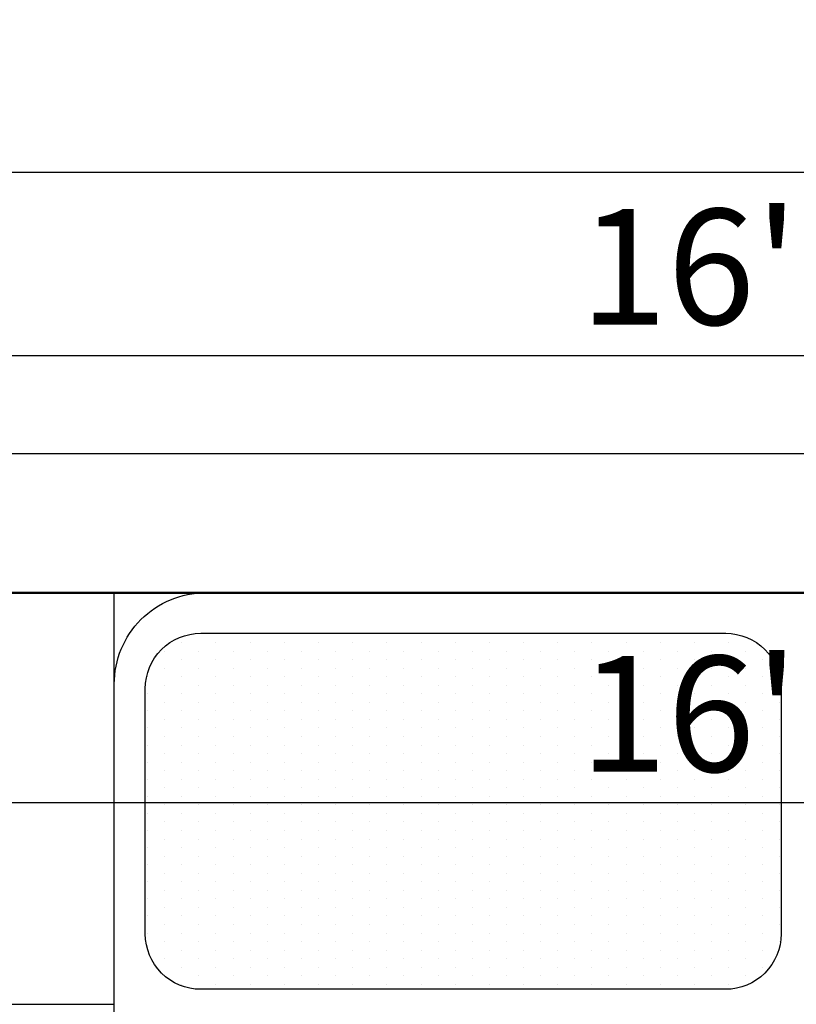
# Model space of a CAD drawing. Units: inches. Extents: x 3064 to 19385, y 846 to 15425.
# Tile 89 of 108: x 7305 to 7338, y 1373 to 1415. Entities that reach past the tile are written whole.
import ezdxf

# ---------------------------------------------------------------- set-up
doc = ezdxf.new("R2010")
doc.units = ezdxf.units.IN
for name, color, linetype, lineweight in [('A-ANNO-DIMS', 2, 'Continuous', 18), ('A-FLOR-FIXT', 9, 'Continuous', 18), ('A-WALL', 7, 'Continuous', 50), ('C-PROP', 6, 'Continuous', 25)]:
    doc.layers.add(name, color=color, linetype=linetype, lineweight=lineweight)
doc.layers.add('BLOCK', color=6, linetype='Continuous')
doc.styles.get("Standard").update_dxf_attribs({"font": 'arial.ttf'})
doc.dimstyles.new('ISO-25', dxfattribs={"dimtxt": 9, "dimasz": 2.5, "dimexe": 1.25, "dimexo": 0.625, "dimtad": 1, "dimdec": 1, "dimlunit": 3, "dimtxsty": 'Standard', "dimcen": 2.5, "dimadec": 0, "dimazin": 0, "dimtfac": 1, "dimtdec": 1, "dimtmove": 0, "dimatfit": 3, "dimfxl": 1, "dimarcsym": 0})

# ---------------------------------------------------------------- blocks, each defined once
blk = doc.blocks.new('*D294')
at = {"layer": 'A-ANNO-DIMS', "color": 0, "lineweight": -2, "transparency": 16777216}
for p, q in [((7240.705, 1396.965), (7240.705, 1401.844)), ((7435.705, 1396.965), (7435.705, 1401.844)), ((7243.205, 1400.594), (7433.205, 1400.594))]:
    blk.add_line(p, q, dxfattribs=at)
at = {"layer": 'A-ANNO-DIMS', "color": 0, "transparency": 16777216}
for points in [[(7243.205, 1401.011), (7243.205, 1400.178), (7240.705, 1400.594)], [(7433.205, 1401.011), (7433.205, 1400.178), (7435.705, 1400.594)]]:
    blk.add_solid(points, dxfattribs=at)
at = {"layer": 'Defpoints', "color": 0, "transparency": 16777216}
for p in [(7435.705, 1400.594), (7240.705, 1396.34), (7435.705, 1396.34)]:
    blk.add_point(p, dxfattribs=at)
at = {"layer": 'A-ANNO-DIMS', "color": 0, "transparency": 16777216, "insert": (7338.205, 1403.774), "char_height": 5, "attachment_point": 5}
blk.add_mtext('16\'-3"', dxfattribs=at)
blk = doc.blocks.new('*D315')
at = {"layer": 'A-ANNO-DIMS', "color": 0, "lineweight": -2, "transparency": 16777216}
for p, q in [((7099.705, 1396.965), (7099.705, 1409.763)), ((7441.705, 1396.965), (7441.705, 1409.763)), ((7102.205, 1408.513), (7439.205, 1408.513))]:
    blk.add_line(p, q, dxfattribs=at)
at = {"layer": 'A-ANNO-DIMS', "color": 0, "transparency": 16777216}
for points in [[(7102.205, 1408.929), (7102.205, 1408.096), (7099.705, 1408.513)], [(7439.205, 1408.929), (7439.205, 1408.096), (7441.705, 1408.513)]]:
    blk.add_solid(points, dxfattribs=at)
at = {"layer": 'Defpoints', "color": 0, "transparency": 16777216}
for p in [(7441.705, 1408.513), (7099.705, 1396.34), (7441.705, 1396.34)]:
    blk.add_point(p, dxfattribs=at)
at = {"layer": 'A-ANNO-DIMS', "color": 0, "transparency": 16777216, "insert": (7270.705, 1411.691), "char_height": 5, "attachment_point": 5}
blk.add_mtext('28\'-6"', dxfattribs=at)
blk = doc.blocks.new('*D290')
at = {"layer": 'A-ANNO-DIMS', "color": 0, "lineweight": -2, "transparency": 16777216}
for p, q in [((7240.705, 1389.715), (7240.705, 1380.039)), ((7435.705, 1389.715), (7435.705, 1380.039)), ((7243.205, 1381.289), (7433.205, 1381.289))]:
    blk.add_line(p, q, dxfattribs=at)
at = {"layer": 'A-ANNO-DIMS', "color": 0, "transparency": 16777216}
for points in [[(7243.205, 1381.705), (7243.205, 1380.872), (7240.705, 1381.289)], [(7433.205, 1381.705), (7433.205, 1380.872), (7435.705, 1381.289)]]:
    blk.add_solid(points, dxfattribs=at)
at = {"layer": 'Defpoints', "color": 0, "transparency": 16777216}
for p in [(7240.705, 1390.34), (7435.705, 1390.34), (7435.705, 1381.289)]:
    blk.add_point(p, dxfattribs=at)
at = {"layer": 'A-ANNO-DIMS', "color": 0, "transparency": 16777216, "insert": (7338.205, 1384.468), "char_height": 5, "attachment_point": 5}
blk.add_mtext('16\'-3"', dxfattribs=at)
blk = doc.blocks.new('*X7')
at = {"color": 0}
for p, q in [((266.25, 456.9375), (266.25, 456.9375)), ((266.4375, 457.03125), (266.4375, 457.03125)), ((266.625, 456.9375), (266.625, 456.9375)), ((266.8125, 457.03125), (266.8125, 457.03125)), ((267, 456.9375), (267, 456.9375)), ((267.1875, 457.03125), (267.1875, 457.03125)), ((267.375, 456.9375), (267.375, 456.9375)), ((267.5625, 457.03125), (267.5625, 457.03125)), ((267.75, 456.9375), (267.75, 456.9375)), ((267.9375, 457.03125), (267.9375, 457.03125)), ((268.125, 456.9375), (268.125, 456.9375)), ((268.3125, 457.03125), (268.3125, 457.03125)), ((268.5, 456.9375), (268.5, 456.9375)), ((268.6875, 457.03125), (268.6875, 457.03125)), ((268.875, 456.9375), (268.875, 456.9375)), ((269.0625, 457.03125), (269.0625, 457.03125)), ((269.25, 456.9375), (269.25, 456.9375)), ((269.4375, 457.03125), (269.4375, 457.03125)), ((269.625, 456.9375), (269.625, 456.9375)), ((269.8125, 457.03125), (269.8125, 457.03125)), ((270, 456.9375), (270, 456.9375)), ((270.1875, 457.03125), (270.1875, 457.03125)), ((270.375, 456.9375), (270.375, 456.9375)), ((270.5625, 457.03125), (270.5625, 457.03125)), ((270.75, 456.9375), (270.75, 456.9375)), ((270.9375, 457.03125), (270.9375, 457.03125)), ((271.125, 456.9375), (271.125, 456.9375)), ((271.3125, 457.03125), (271.3125, 457.03125)), ((271.5, 456.9375), (271.5, 456.9375)), ((271.6875, 457.03125), (271.6875, 457.03125)), ((271.875, 456.9375), (271.875, 456.9375)), ((272.0625, 457.03125), (272.0625, 457.03125)), ((272.25, 456.9375), (272.25, 456.9375)), ((266.0625, 456.84375), (266.0625, 456.84375)), ((266.4375, 456.84375), (266.4375, 456.84375)), ((266.8125, 456.84375), (266.8125, 456.84375)), ((267.1875, 456.84375), (267.1875, 456.84375)), ((267.5625, 456.84375), (267.5625, 456.84375)), ((267.9375, 456.84375), (267.9375, 456.84375)), ((268.3125, 456.84375), (268.3125, 456.84375)), ((268.6875, 456.84375), (268.6875, 456.84375)), ((269.0625, 456.84375), (269.0625, 456.84375)), ((269.4375, 456.84375), (269.4375, 456.84375)), ((269.8125, 456.84375), (269.8125, 456.84375)), ((270.1875, 456.84375), (270.1875, 456.84375)), ((270.5625, 456.84375), (270.5625, 456.84375)), ((270.9375, 456.84375), (270.9375, 456.84375)), ((271.3125, 456.84375), (271.3125, 456.84375)), ((271.6875, 456.84375), (271.6875, 456.84375)), ((272.0625, 456.84375), (272.0625, 456.84375)), ((272.4375, 456.84375), (272.4375, 456.84375)), ((266.25, 456.75), (266.25, 456.75)), ((266.625, 456.75), (266.625, 456.75)), ((267, 456.75), (267, 456.75)), ((267.375, 456.75), (267.375, 456.75)), ((267.75, 456.75), (267.75, 456.75)), ((268.125, 456.75), (268.125, 456.75)), ((268.5, 456.75), (268.5, 456.75)), ((268.875, 456.75), (268.875, 456.75)), ((269.25, 456.75), (269.25, 456.75)), ((269.625, 456.75), (269.625, 456.75)), ((270, 456.75), (270, 456.75)), ((270.375, 456.75), (270.375, 456.75)), ((270.75, 456.75), (270.75, 456.75)), ((271.125, 456.75), (271.125, 456.75)), ((271.5, 456.75), (271.5, 456.75)), ((271.875, 456.75), (271.875, 456.75)), ((272.25, 456.75), (272.25, 456.75)), ((272.625, 456.75), (272.625, 456.75)), ((266.0625, 456.65625), (266.0625, 456.65625)), ((266.4375, 456.65625), (266.4375, 456.65625)), ((266.8125, 456.65625), (266.8125, 456.65625)), ((267.1875, 456.65625), (267.1875, 456.65625)), ((267.5625, 456.65625), (267.5625, 456.65625)), ((267.9375, 456.65625), (267.9375, 456.65625)), ((268.3125, 456.65625), (268.3125, 456.65625)), ((268.6875, 456.65625), (268.6875, 456.65625)), ((269.0625, 456.65625), (269.0625, 456.65625)), ((269.4375, 456.65625), (269.4375, 456.65625)), ((269.8125, 456.65625), (269.8125, 456.65625)), ((270.1875, 456.65625), (270.1875, 456.65625)), ((270.5625, 456.65625), (270.5625, 456.65625)), ((270.9375, 456.65625), (270.9375, 456.65625)), ((271.3125, 456.65625), (271.3125, 456.65625)), ((271.6875, 456.65625), (271.6875, 456.65625)), ((272.0625, 456.65625), (272.0625, 456.65625)), ((272.4375, 456.65625), (272.4375, 456.65625)), ((265.875, 456.5625), (265.875, 456.5625)), ((266.25, 456.5625), (266.25, 456.5625)), ((266.625, 456.5625), (266.625, 456.5625)), ((267, 456.5625), (267, 456.5625)), ((267.375, 456.5625), (267.375, 456.5625)), ((267.75, 456.5625), (267.75, 456.5625)), ((268.125, 456.5625), (268.125, 456.5625)), ((268.5, 456.5625), (268.5, 456.5625)), ((268.875, 456.5625), (268.875, 456.5625)), ((269.25, 456.5625), (269.25, 456.5625)), ((269.625, 456.5625), (269.625, 456.5625)), ((270, 456.5625), (270, 456.5625)), ((270.375, 456.5625), (270.375, 456.5625)), ((270.75, 456.5625), (270.75, 456.5625)), ((271.125, 456.5625), (271.125, 456.5625)), ((271.5, 456.5625), (271.5, 456.5625)), ((271.875, 456.5625), (271.875, 456.5625)), ((272.25, 456.5625), (272.25, 456.5625)), ((272.625, 456.5625), (272.625, 456.5625)), ((266.0625, 456.46875), (266.0625, 456.46875)), ((266.4375, 456.46875), (266.4375, 456.46875)), ((266.8125, 456.46875), (266.8125, 456.46875)), ((267.1875, 456.46875), (267.1875, 456.46875)), ((267.5625, 456.46875), (267.5625, 456.46875)), ((267.9375, 456.46875), (267.9375, 456.46875)), ((268.3125, 456.46875), (268.3125, 456.46875)), ((268.6875, 456.46875), (268.6875, 456.46875)), ((269.0625, 456.46875), (269.0625, 456.46875)), ((269.4375, 456.46875), (269.4375, 456.46875)), ((269.8125, 456.46875), (269.8125, 456.46875)), ((270.1875, 456.46875), (270.1875, 456.46875)), ((270.5625, 456.46875), (270.5625, 456.46875)), ((270.9375, 456.46875), (270.9375, 456.46875)), ((271.3125, 456.46875), (271.3125, 456.46875)), ((271.6875, 456.46875), (271.6875, 456.46875)), ((272.0625, 456.46875), (272.0625, 456.46875)), ((272.4375, 456.46875), (272.4375, 456.46875)), ((272.8125, 456.46875), (272.8125, 456.46875)), ((265.875, 456.375), (265.875, 456.375)), ((266.25, 456.375), (266.25, 456.375)), ((266.625, 456.375), (266.625, 456.375)), ((267, 456.375), (267, 456.375)), ((267.375, 456.375), (267.375, 456.375)), ((267.75, 456.375), (267.75, 456.375)), ((268.125, 456.375), (268.125, 456.375)), ((268.5, 456.375), (268.5, 456.375)), ((268.875, 456.375), (268.875, 456.375)), ((269.25, 456.375), (269.25, 456.375)), ((269.625, 456.375), (269.625, 456.375)), ((270, 456.375), (270, 456.375)), ((270.375, 456.375), (270.375, 456.375)), ((270.75, 456.375), (270.75, 456.375)), ((271.125, 456.375), (271.125, 456.375)), ((271.5, 456.375), (271.5, 456.375)), ((271.875, 456.375), (271.875, 456.375)), ((272.25, 456.375), (272.25, 456.375)), ((272.625, 456.375), (272.625, 456.375)), ((265.875, 456.1875), (265.875, 456.1875)), ((266.0625, 456.28125), (266.0625, 456.28125)), ((266.25, 456.1875), (266.25, 456.1875)), ((266.4375, 456.28125), (266.4375, 456.28125)), ((266.625, 456.1875), (266.625, 456.1875)), ((266.8125, 456.28125), (266.8125, 456.28125)), ((267, 456.1875), (267, 456.1875)), ((267.1875, 456.28125), (267.1875, 456.28125)), ((267.375, 456.1875), (267.375, 456.1875)), ((267.5625, 456.28125), (267.5625, 456.28125)), ((267.75, 456.1875), (267.75, 456.1875)), ((267.9375, 456.28125), (267.9375, 456.28125)), ((268.125, 456.1875), (268.125, 456.1875)), ((268.3125, 456.28125), (268.3125, 456.28125)), ((268.5, 456.1875), (268.5, 456.1875)), ((268.6875, 456.28125), (268.6875, 456.28125)), ((268.875, 456.1875), (268.875, 456.1875)), ((269.0625, 456.28125), (269.0625, 456.28125)), ((269.25, 456.1875), (269.25, 456.1875)), ((269.4375, 456.28125), (269.4375, 456.28125)), ((269.625, 456.1875), (269.625, 456.1875)), ((269.8125, 456.28125), (269.8125, 456.28125)), ((270, 456.1875), (270, 456.1875)), ((270.1875, 456.28125), (270.1875, 456.28125)), ((270.375, 456.1875), (270.375, 456.1875)), ((270.5625, 456.28125), (270.5625, 456.28125)), ((270.75, 456.1875), (270.75, 456.1875)), ((270.9375, 456.28125), (270.9375, 456.28125)), ((271.125, 456.1875), (271.125, 456.1875)), ((271.3125, 456.28125), (271.3125, 456.28125)), ((271.5, 456.1875), (271.5, 456.1875)), ((271.6875, 456.28125), (271.6875, 456.28125)), ((271.875, 456.1875), (271.875, 456.1875)), ((272.0625, 456.28125), (272.0625, 456.28125)), ((272.25, 456.1875), (272.25, 456.1875)), ((272.4375, 456.28125), (272.4375, 456.28125)), ((272.625, 456.1875), (272.625, 456.1875)), ((272.8125, 456.28125), (272.8125, 456.28125)), ((266.0625, 456.09375), (266.0625, 456.09375)), ((266.4375, 456.09375), (266.4375, 456.09375)), ((266.8125, 456.09375), (266.8125, 456.09375)), ((267.1875, 456.09375), (267.1875, 456.09375)), ((267.5625, 456.09375), (267.5625, 456.09375)), ((267.9375, 456.09375), (267.9375, 456.09375)), ((268.3125, 456.09375), (268.3125, 456.09375)), ((268.6875, 456.09375), (268.6875, 456.09375)), ((269.0625, 456.09375), (269.0625, 456.09375)), ((269.4375, 456.09375), (269.4375, 456.09375)), ((269.8125, 456.09375), (269.8125, 456.09375)), ((270.1875, 456.09375), (270.1875, 456.09375)), ((270.5625, 456.09375), (270.5625, 456.09375)), ((270.9375, 456.09375), (270.9375, 456.09375)), ((271.3125, 456.09375), (271.3125, 456.09375)), ((271.6875, 456.09375), (271.6875, 456.09375)), ((272.0625, 456.09375), (272.0625, 456.09375)), ((272.4375, 456.09375), (272.4375, 456.09375)), ((272.8125, 456.09375), (272.8125, 456.09375)), ((265.875, 456), (265.875, 456)), ((266.25, 456), (266.25, 456)), ((266.625, 456), (266.625, 456)), ((267, 456), (267, 456)), ((267.375, 456), (267.375, 456)), ((267.75, 456), (267.75, 456)), ((268.125, 456), (268.125, 456)), ((268.5, 456), (268.5, 456)), ((268.875, 456), (268.875, 456)), ((269.25, 456), (269.25, 456)), ((269.625, 456), (269.625, 456)), ((270, 456), (270, 456)), ((270.375, 456), (270.375, 456)), ((270.75, 456), (270.75, 456)), ((271.125, 456), (271.125, 456)), ((271.5, 456), (271.5, 456)), ((271.875, 456), (271.875, 456)), ((272.25, 456), (272.25, 456)), ((272.625, 456), (272.625, 456)), ((266.0625, 455.90625), (266.0625, 455.90625)), ((266.4375, 455.90625), (266.4375, 455.90625)), ((266.8125, 455.90625), (266.8125, 455.90625)), ((267.1875, 455.90625), (267.1875, 455.90625)), ((267.5625, 455.90625), (267.5625, 455.90625)), ((267.9375, 455.90625), (267.9375, 455.90625)), ((268.3125, 455.90625), (268.3125, 455.90625)), ((268.6875, 455.90625), (268.6875, 455.90625)), ((269.0625, 455.90625), (269.0625, 455.90625)), ((269.4375, 455.90625), (269.4375, 455.90625)), ((269.8125, 455.90625), (269.8125, 455.90625)), ((270.1875, 455.90625), (270.1875, 455.90625)), ((270.5625, 455.90625), (270.5625, 455.90625)), ((270.9375, 455.90625), (270.9375, 455.90625)), ((271.3125, 455.90625), (271.3125, 455.90625)), ((271.6875, 455.90625), (271.6875, 455.90625)), ((272.0625, 455.90625), (272.0625, 455.90625)), ((272.4375, 455.90625), (272.4375, 455.90625)), ((272.8125, 455.90625), (272.8125, 455.90625)), ((265.875, 455.8125), (265.875, 455.8125)), ((266.25, 455.8125), (266.25, 455.8125)), ((266.625, 455.8125), (266.625, 455.8125)), ((267, 455.8125), (267, 455.8125)), ((267.375, 455.8125), (267.375, 455.8125)), ((267.75, 455.8125), (267.75, 455.8125)), ((268.125, 455.8125), (268.125, 455.8125)), ((268.5, 455.8125), (268.5, 455.8125)), ((268.875, 455.8125), (268.875, 455.8125)), ((269.25, 455.8125), (269.25, 455.8125)), ((269.625, 455.8125), (269.625, 455.8125)), ((270, 455.8125), (270, 455.8125)), ((270.375, 455.8125), (270.375, 455.8125)), ((270.75, 455.8125), (270.75, 455.8125)), ((271.125, 455.8125), (271.125, 455.8125)), ((271.5, 455.8125), (271.5, 455.8125)), ((271.875, 455.8125), (271.875, 455.8125)), ((272.25, 455.8125), (272.25, 455.8125)), ((272.625, 455.8125), (272.625, 455.8125)), ((266.0625, 455.71875), (266.0625, 455.71875)), ((266.4375, 455.71875), (266.4375, 455.71875)), ((266.8125, 455.71875), (266.8125, 455.71875)), ((267.1875, 455.71875), (267.1875, 455.71875)), ((267.5625, 455.71875), (267.5625, 455.71875)), ((267.9375, 455.71875), (267.9375, 455.71875)), ((268.3125, 455.71875), (268.3125, 455.71875)), ((268.6875, 455.71875), (268.6875, 455.71875)), ((269.0625, 455.71875), (269.0625, 455.71875)), ((269.4375, 455.71875), (269.4375, 455.71875)), ((269.8125, 455.71875), (269.8125, 455.71875)), ((270.1875, 455.71875), (270.1875, 455.71875)), ((270.5625, 455.71875), (270.5625, 455.71875)), ((270.9375, 455.71875), (270.9375, 455.71875)), ((271.3125, 455.71875), (271.3125, 455.71875)), ((271.6875, 455.71875), (271.6875, 455.71875)), ((272.0625, 455.71875), (272.0625, 455.71875)), ((272.4375, 455.71875), (272.4375, 455.71875)), ((272.8125, 455.71875), (272.8125, 455.71875)), ((265.875, 455.625), (265.875, 455.625)), ((266.0625, 455.53125), (266.0625, 455.53125)), ((266.25, 455.625), (266.25, 455.625)), ((266.4375, 455.53125), (266.4375, 455.53125)), ((266.625, 455.625), (266.625, 455.625)), ((266.8125, 455.53125), (266.8125, 455.53125)), ((267, 455.625), (267, 455.625)), ((267.1875, 455.53125), (267.1875, 455.53125)), ((267.375, 455.625), (267.375, 455.625)), ((267.5625, 455.53125), (267.5625, 455.53125)), ((267.75, 455.625), (267.75, 455.625)), ((267.9375, 455.53125), (267.9375, 455.53125)), ((268.125, 455.625), (268.125, 455.625)), ((268.3125, 455.53125), (268.3125, 455.53125)), ((268.5, 455.625), (268.5, 455.625)), ((268.6875, 455.53125), (268.6875, 455.53125)), ((268.875, 455.625), (268.875, 455.625)), ((269.0625, 455.53125), (269.0625, 455.53125)), ((269.25, 455.625), (269.25, 455.625)), ((269.4375, 455.53125), (269.4375, 455.53125)), ((269.625, 455.625), (269.625, 455.625)), ((269.8125, 455.53125), (269.8125, 455.53125)), ((270, 455.625), (270, 455.625)), ((270.1875, 455.53125), (270.1875, 455.53125)), ((270.375, 455.625), (270.375, 455.625)), ((270.5625, 455.53125), (270.5625, 455.53125)), ((270.75, 455.625), (270.75, 455.625)), ((270.9375, 455.53125), (270.9375, 455.53125)), ((271.125, 455.625), (271.125, 455.625)), ((271.3125, 455.53125), (271.3125, 455.53125)), ((271.5, 455.625), (271.5, 455.625)), ((271.6875, 455.53125), (271.6875, 455.53125)), ((271.875, 455.625), (271.875, 455.625)), ((272.0625, 455.53125), (272.0625, 455.53125)), ((272.25, 455.625), (272.25, 455.625)), ((272.4375, 455.53125), (272.4375, 455.53125)), ((272.625, 455.625), (272.625, 455.625)), ((272.8125, 455.53125), (272.8125, 455.53125)), ((265.875, 455.4375), (265.875, 455.4375)), ((266.25, 455.4375), (266.25, 455.4375)), ((266.625, 455.4375), (266.625, 455.4375)), ((267, 455.4375), (267, 455.4375)), ((267.375, 455.4375), (267.375, 455.4375)), ((267.75, 455.4375), (267.75, 455.4375)), ((268.125, 455.4375), (268.125, 455.4375)), ((268.5, 455.4375), (268.5, 455.4375)), ((268.875, 455.4375), (268.875, 455.4375)), ((269.25, 455.4375), (269.25, 455.4375)), ((269.625, 455.4375), (269.625, 455.4375)), ((270, 455.4375), (270, 455.4375)), ((270.375, 455.4375), (270.375, 455.4375)), ((270.75, 455.4375), (270.75, 455.4375)), ((271.125, 455.4375), (271.125, 455.4375)), ((271.5, 455.4375), (271.5, 455.4375)), ((271.875, 455.4375), (271.875, 455.4375)), ((272.25, 455.4375), (272.25, 455.4375)), ((272.625, 455.4375), (272.625, 455.4375)), ((266.0625, 455.34375), (266.0625, 455.34375)), ((266.4375, 455.34375), (266.4375, 455.34375)), ((266.8125, 455.34375), (266.8125, 455.34375)), ((267.1875, 455.34375), (267.1875, 455.34375)), ((267.5625, 455.34375), (267.5625, 455.34375)), ((267.9375, 455.34375), (267.9375, 455.34375)), ((268.3125, 455.34375), (268.3125, 455.34375)), ((268.6875, 455.34375), (268.6875, 455.34375)), ((269.0625, 455.34375), (269.0625, 455.34375)), ((269.4375, 455.34375), (269.4375, 455.34375)), ((269.8125, 455.34375), (269.8125, 455.34375)), ((270.1875, 455.34375), (270.1875, 455.34375)), ((270.5625, 455.34375), (270.5625, 455.34375)), ((270.9375, 455.34375), (270.9375, 455.34375)), ((271.3125, 455.34375), (271.3125, 455.34375)), ((271.6875, 455.34375), (271.6875, 455.34375)), ((272.0625, 455.34375), (272.0625, 455.34375)), ((272.4375, 455.34375), (272.4375, 455.34375)), ((272.8125, 455.34375), (272.8125, 455.34375)), ((265.875, 455.25), (265.875, 455.25)), ((266.25, 455.25), (266.25, 455.25)), ((266.625, 455.25), (266.625, 455.25)), ((267, 455.25), (267, 455.25)), ((267.375, 455.25), (267.375, 455.25)), ((267.75, 455.25), (267.75, 455.25)), ((268.125, 455.25), (268.125, 455.25)), ((268.5, 455.25), (268.5, 455.25)), ((268.875, 455.25), (268.875, 455.25)), ((269.25, 455.25), (269.25, 455.25)), ((269.625, 455.25), (269.625, 455.25)), ((270, 455.25), (270, 455.25)), ((270.375, 455.25), (270.375, 455.25)), ((270.75, 455.25), (270.75, 455.25)), ((271.125, 455.25), (271.125, 455.25)), ((271.5, 455.25), (271.5, 455.25)), ((271.875, 455.25), (271.875, 455.25)), ((272.25, 455.25), (272.25, 455.25)), ((272.625, 455.25), (272.625, 455.25)), ((266.0625, 455.15625), (266.0625, 455.15625)), ((266.4375, 455.15625), (266.4375, 455.15625)), ((266.8125, 455.15625), (266.8125, 455.15625)), ((267.1875, 455.15625), (267.1875, 455.15625)), ((267.5625, 455.15625), (267.5625, 455.15625)), ((267.9375, 455.15625), (267.9375, 455.15625)), ((268.3125, 455.15625), (268.3125, 455.15625)), ((268.6875, 455.15625), (268.6875, 455.15625)), ((269.0625, 455.15625), (269.0625, 455.15625)), ((269.4375, 455.15625), (269.4375, 455.15625)), ((269.8125, 455.15625), (269.8125, 455.15625)), ((270.1875, 455.15625), (270.1875, 455.15625)), ((270.5625, 455.15625), (270.5625, 455.15625)), ((270.9375, 455.15625), (270.9375, 455.15625)), ((271.3125, 455.15625), (271.3125, 455.15625)), ((271.6875, 455.15625), (271.6875, 455.15625)), ((272.0625, 455.15625), (272.0625, 455.15625)), ((272.4375, 455.15625), (272.4375, 455.15625)), ((272.8125, 455.15625), (272.8125, 455.15625)), ((265.875, 455.0625), (265.875, 455.0625)), ((266.25, 455.0625), (266.25, 455.0625)), ((266.625, 455.0625), (266.625, 455.0625)), ((267, 455.0625), (267, 455.0625)), ((267.375, 455.0625), (267.375, 455.0625)), ((267.75, 455.0625), (267.75, 455.0625)), ((268.125, 455.0625), (268.125, 455.0625)), ((268.5, 455.0625), (268.5, 455.0625)), ((268.875, 455.0625), (268.875, 455.0625)), ((269.25, 455.0625), (269.25, 455.0625)), ((269.625, 455.0625), (269.625, 455.0625)), ((270, 455.0625), (270, 455.0625)), ((270.375, 455.0625), (270.375, 455.0625)), ((270.75, 455.0625), (270.75, 455.0625)), ((271.125, 455.0625), (271.125, 455.0625)), ((271.5, 455.0625), (271.5, 455.0625)), ((271.875, 455.0625), (271.875, 455.0625)), ((272.25, 455.0625), (272.25, 455.0625)), ((272.625, 455.0625), (272.625, 455.0625)), ((266.0625, 454.96875), (266.0625, 454.96875)), ((266.4375, 454.96875), (266.4375, 454.96875)), ((266.8125, 454.96875), (266.8125, 454.96875)), ((267.1875, 454.96875), (267.1875, 454.96875)), ((267.5625, 454.96875), (267.5625, 454.96875)), ((267.9375, 454.96875), (267.9375, 454.96875)), ((268.3125, 454.96875), (268.3125, 454.96875)), ((268.6875, 454.96875), (268.6875, 454.96875)), ((269.0625, 454.96875), (269.0625, 454.96875)), ((269.4375, 454.96875), (269.4375, 454.96875)), ((269.8125, 454.96875), (269.8125, 454.96875)), ((270.1875, 454.96875), (270.1875, 454.96875)), ((270.5625, 454.96875), (270.5625, 454.96875)), ((270.9375, 454.96875), (270.9375, 454.96875)), ((271.3125, 454.96875), (271.3125, 454.96875)), ((271.6875, 454.96875), (271.6875, 454.96875)), ((272.0625, 454.96875), (272.0625, 454.96875)), ((272.4375, 454.96875), (272.4375, 454.96875)), ((272.8125, 454.96875), (272.8125, 454.96875)), ((265.875, 454.875), (265.875, 454.875)), ((266.0625, 454.78125), (266.0625, 454.78125)), ((266.25, 454.875), (266.25, 454.875)), ((266.4375, 454.78125), (266.4375, 454.78125)), ((266.625, 454.875), (266.625, 454.875)), ((266.8125, 454.78125), (266.8125, 454.78125)), ((267, 454.875), (267, 454.875)), ((267.1875, 454.78125), (267.1875, 454.78125)), ((267.375, 454.875), (267.375, 454.875)), ((267.5625, 454.78125), (267.5625, 454.78125)), ((267.75, 454.875), (267.75, 454.875)), ((267.9375, 454.78125), (267.9375, 454.78125)), ((268.125, 454.875), (268.125, 454.875)), ((268.3125, 454.78125), (268.3125, 454.78125)), ((268.5, 454.875), (268.5, 454.875)), ((268.6875, 454.78125), (268.6875, 454.78125)), ((268.875, 454.875), (268.875, 454.875)), ((269.0625, 454.78125), (269.0625, 454.78125)), ((269.25, 454.875), (269.25, 454.875)), ((269.4375, 454.78125), (269.4375, 454.78125)), ((269.625, 454.875), (269.625, 454.875)), ((269.8125, 454.78125), (269.8125, 454.78125)), ((270, 454.875), (270, 454.875)), ((270.1875, 454.78125), (270.1875, 454.78125)), ((270.375, 454.875), (270.375, 454.875)), ((270.5625, 454.78125), (270.5625, 454.78125)), ((270.75, 454.875), (270.75, 454.875)), ((270.9375, 454.78125), (270.9375, 454.78125)), ((271.125, 454.875), (271.125, 454.875)), ((271.3125, 454.78125), (271.3125, 454.78125)), ((271.5, 454.875), (271.5, 454.875)), ((271.6875, 454.78125), (271.6875, 454.78125)), ((271.875, 454.875), (271.875, 454.875)), ((272.0625, 454.78125), (272.0625, 454.78125)), ((272.25, 454.875), (272.25, 454.875)), ((272.4375, 454.78125), (272.4375, 454.78125)), ((272.625, 454.875), (272.625, 454.875)), ((272.8125, 454.78125), (272.8125, 454.78125)), ((265.875, 454.6875), (265.875, 454.6875)), ((266.25, 454.6875), (266.25, 454.6875)), ((266.625, 454.6875), (266.625, 454.6875)), ((267, 454.6875), (267, 454.6875)), ((267.375, 454.6875), (267.375, 454.6875)), ((267.75, 454.6875), (267.75, 454.6875)), ((268.125, 454.6875), (268.125, 454.6875)), ((268.5, 454.6875), (268.5, 454.6875)), ((268.875, 454.6875), (268.875, 454.6875)), ((269.25, 454.6875), (269.25, 454.6875)), ((269.625, 454.6875), (269.625, 454.6875)), ((270, 454.6875), (270, 454.6875)), ((270.375, 454.6875), (270.375, 454.6875)), ((270.75, 454.6875), (270.75, 454.6875)), ((271.125, 454.6875), (271.125, 454.6875)), ((271.5, 454.6875), (271.5, 454.6875)), ((271.875, 454.6875), (271.875, 454.6875)), ((272.25, 454.6875), (272.25, 454.6875)), ((272.625, 454.6875), (272.625, 454.6875)), ((266.0625, 454.59375), (266.0625, 454.59375)), ((266.4375, 454.59375), (266.4375, 454.59375)), ((266.8125, 454.59375), (266.8125, 454.59375)), ((267.1875, 454.59375), (267.1875, 454.59375)), ((267.5625, 454.59375), (267.5625, 454.59375)), ((267.9375, 454.59375), (267.9375, 454.59375)), ((268.3125, 454.59375), (268.3125, 454.59375)), ((268.6875, 454.59375), (268.6875, 454.59375)), ((269.0625, 454.59375), (269.0625, 454.59375)), ((269.4375, 454.59375), (269.4375, 454.59375)), ((269.8125, 454.59375), (269.8125, 454.59375)), ((270.1875, 454.59375), (270.1875, 454.59375)), ((270.5625, 454.59375), (270.5625, 454.59375)), ((270.9375, 454.59375), (270.9375, 454.59375)), ((271.3125, 454.59375), (271.3125, 454.59375)), ((271.6875, 454.59375), (271.6875, 454.59375)), ((272.0625, 454.59375), (272.0625, 454.59375)), ((272.4375, 454.59375), (272.4375, 454.59375)), ((272.8125, 454.59375), (272.8125, 454.59375)), ((265.875, 454.5), (265.875, 454.5)), ((266.25, 454.5), (266.25, 454.5)), ((266.625, 454.5), (266.625, 454.5)), ((267, 454.5), (267, 454.5)), ((267.375, 454.5), (267.375, 454.5)), ((267.75, 454.5), (267.75, 454.5)), ((268.125, 454.5), (268.125, 454.5)), ((268.5, 454.5), (268.5, 454.5)), ((268.875, 454.5), (268.875, 454.5)), ((269.25, 454.5), (269.25, 454.5)), ((269.625, 454.5), (269.625, 454.5)), ((270, 454.5), (270, 454.5)), ((270.375, 454.5), (270.375, 454.5)), ((270.75, 454.5), (270.75, 454.5)), ((271.125, 454.5), (271.125, 454.5)), ((271.5, 454.5), (271.5, 454.5)), ((271.875, 454.5), (271.875, 454.5)), ((272.25, 454.5), (272.25, 454.5)), ((272.625, 454.5), (272.625, 454.5)), ((266.0625, 454.40625), (266.0625, 454.40625)), ((266.4375, 454.40625), (266.4375, 454.40625)), ((266.8125, 454.40625), (266.8125, 454.40625)), ((267.1875, 454.40625), (267.1875, 454.40625)), ((267.5625, 454.40625), (267.5625, 454.40625)), ((267.9375, 454.40625), (267.9375, 454.40625)), ((268.3125, 454.40625), (268.3125, 454.40625)), ((268.6875, 454.40625), (268.6875, 454.40625)), ((269.0625, 454.40625), (269.0625, 454.40625)), ((269.4375, 454.40625), (269.4375, 454.40625)), ((269.8125, 454.40625), (269.8125, 454.40625)), ((270.1875, 454.40625), (270.1875, 454.40625)), ((270.5625, 454.40625), (270.5625, 454.40625)), ((270.9375, 454.40625), (270.9375, 454.40625)), ((271.3125, 454.40625), (271.3125, 454.40625)), ((271.6875, 454.40625), (271.6875, 454.40625)), ((272.0625, 454.40625), (272.0625, 454.40625)), ((272.4375, 454.40625), (272.4375, 454.40625)), ((272.8125, 454.40625), (272.8125, 454.40625)), ((265.875, 454.3125), (265.875, 454.3125)), ((266.25, 454.3125), (266.25, 454.3125)), ((266.625, 454.3125), (266.625, 454.3125)), ((267, 454.3125), (267, 454.3125)), ((267.375, 454.3125), (267.375, 454.3125)), ((267.75, 454.3125), (267.75, 454.3125)), ((268.125, 454.3125), (268.125, 454.3125)), ((268.5, 454.3125), (268.5, 454.3125)), ((268.875, 454.3125), (268.875, 454.3125)), ((269.25, 454.3125), (269.25, 454.3125)), ((269.625, 454.3125), (269.625, 454.3125)), ((270, 454.3125), (270, 454.3125)), ((270.375, 454.3125), (270.375, 454.3125)), ((270.75, 454.3125), (270.75, 454.3125)), ((271.125, 454.3125), (271.125, 454.3125)), ((271.5, 454.3125), (271.5, 454.3125)), ((271.875, 454.3125), (271.875, 454.3125)), ((272.25, 454.3125), (272.25, 454.3125)), ((272.625, 454.3125), (272.625, 454.3125)), ((266.0625, 454.21875), (266.0625, 454.21875)), ((266.4375, 454.21875), (266.4375, 454.21875)), ((266.8125, 454.21875), (266.8125, 454.21875)), ((267.1875, 454.21875), (267.1875, 454.21875)), ((267.5625, 454.21875), (267.5625, 454.21875)), ((267.9375, 454.21875), (267.9375, 454.21875)), ((268.3125, 454.21875), (268.3125, 454.21875)), ((268.6875, 454.21875), (268.6875, 454.21875)), ((269.0625, 454.21875), (269.0625, 454.21875)), ((269.4375, 454.21875), (269.4375, 454.21875)), ((269.8125, 454.21875), (269.8125, 454.21875)), ((270.1875, 454.21875), (270.1875, 454.21875)), ((270.5625, 454.21875), (270.5625, 454.21875)), ((270.9375, 454.21875), (270.9375, 454.21875)), ((271.3125, 454.21875), (271.3125, 454.21875)), ((271.6875, 454.21875), (271.6875, 454.21875)), ((272.0625, 454.21875), (272.0625, 454.21875)), ((272.4375, 454.21875), (272.4375, 454.21875)), ((272.8125, 454.21875), (272.8125, 454.21875)), ((265.875, 454.125), (265.875, 454.125)), ((266.0625, 454.03125), (266.0625, 454.03125)), ((266.25, 454.125), (266.25, 454.125)), ((266.4375, 454.03125), (266.4375, 454.03125)), ((266.625, 454.125), (266.625, 454.125)), ((266.8125, 454.03125), (266.8125, 454.03125)), ((267, 454.125), (267, 454.125)), ((267.1875, 454.03125), (267.1875, 454.03125)), ((267.375, 454.125), (267.375, 454.125)), ((267.5625, 454.03125), (267.5625, 454.03125)), ((267.75, 454.125), (267.75, 454.125)), ((267.9375, 454.03125), (267.9375, 454.03125)), ((268.125, 454.125), (268.125, 454.125)), ((268.3125, 454.03125), (268.3125, 454.03125)), ((268.5, 454.125), (268.5, 454.125)), ((268.6875, 454.03125), (268.6875, 454.03125)), ((268.875, 454.125), (268.875, 454.125)), ((269.0625, 454.03125), (269.0625, 454.03125)), ((269.25, 454.125), (269.25, 454.125)), ((269.4375, 454.03125), (269.4375, 454.03125)), ((269.625, 454.125), (269.625, 454.125)), ((269.8125, 454.03125), (269.8125, 454.03125)), ((270, 454.125), (270, 454.125)), ((270.1875, 454.03125), (270.1875, 454.03125)), ((270.375, 454.125), (270.375, 454.125)), ((270.5625, 454.03125), (270.5625, 454.03125)), ((270.75, 454.125), (270.75, 454.125)), ((270.9375, 454.03125), (270.9375, 454.03125)), ((271.125, 454.125), (271.125, 454.125)), ((271.3125, 454.03125), (271.3125, 454.03125)), ((271.5, 454.125), (271.5, 454.125)), ((271.6875, 454.03125), (271.6875, 454.03125)), ((271.875, 454.125), (271.875, 454.125)), ((272.0625, 454.03125), (272.0625, 454.03125)), ((272.25, 454.125), (272.25, 454.125)), ((272.4375, 454.03125), (272.4375, 454.03125)), ((272.625, 454.125), (272.625, 454.125)), ((272.8125, 454.03125), (272.8125, 454.03125)), ((265.875, 453.9375), (265.875, 453.9375)), ((266.25, 453.9375), (266.25, 453.9375)), ((266.625, 453.9375), (266.625, 453.9375)), ((267, 453.9375), (267, 453.9375)), ((267.375, 453.9375), (267.375, 453.9375)), ((267.75, 453.9375), (267.75, 453.9375)), ((268.125, 453.9375), (268.125, 453.9375)), ((268.5, 453.9375), (268.5, 453.9375)), ((268.875, 453.9375), (268.875, 453.9375)), ((269.25, 453.9375), (269.25, 453.9375)), ((269.625, 453.9375), (269.625, 453.9375)), ((270, 453.9375), (270, 453.9375)), ((270.375, 453.9375), (270.375, 453.9375)), ((270.75, 453.9375), (270.75, 453.9375)), ((271.125, 453.9375), (271.125, 453.9375)), ((271.5, 453.9375), (271.5, 453.9375)), ((271.875, 453.9375), (271.875, 453.9375)), ((272.25, 453.9375), (272.25, 453.9375)), ((272.625, 453.9375), (272.625, 453.9375)), ((266.0625, 453.84375), (266.0625, 453.84375)), ((266.4375, 453.84375), (266.4375, 453.84375)), ((266.8125, 453.84375), (266.8125, 453.84375)), ((267.1875, 453.84375), (267.1875, 453.84375)), ((267.5625, 453.84375), (267.5625, 453.84375)), ((267.9375, 453.84375), (267.9375, 453.84375)), ((268.3125, 453.84375), (268.3125, 453.84375)), ((268.6875, 453.84375), (268.6875, 453.84375)), ((269.0625, 453.84375), (269.0625, 453.84375)), ((269.4375, 453.84375), (269.4375, 453.84375)), ((269.8125, 453.84375), (269.8125, 453.84375)), ((270.1875, 453.84375), (270.1875, 453.84375)), ((270.5625, 453.84375), (270.5625, 453.84375)), ((270.9375, 453.84375), (270.9375, 453.84375)), ((271.3125, 453.84375), (271.3125, 453.84375)), ((271.6875, 453.84375), (271.6875, 453.84375)), ((272.0625, 453.84375), (272.0625, 453.84375)), ((272.4375, 453.84375), (272.4375, 453.84375)), ((272.8125, 453.84375), (272.8125, 453.84375)), ((265.875, 453.75), (265.875, 453.75)), ((266.25, 453.75), (266.25, 453.75)), ((266.625, 453.75), (266.625, 453.75)), ((267, 453.75), (267, 453.75)), ((267.375, 453.75), (267.375, 453.75)), ((267.75, 453.75), (267.75, 453.75)), ((268.125, 453.75), (268.125, 453.75)), ((268.5, 453.75), (268.5, 453.75)), ((268.875, 453.75), (268.875, 453.75)), ((269.25, 453.75), (269.25, 453.75)), ((269.625, 453.75), (269.625, 453.75)), ((270, 453.75), (270, 453.75)), ((270.375, 453.75), (270.375, 453.75)), ((270.75, 453.75), (270.75, 453.75)), ((271.125, 453.75), (271.125, 453.75)), ((271.5, 453.75), (271.5, 453.75)), ((271.875, 453.75), (271.875, 453.75)), ((272.25, 453.75), (272.25, 453.75)), ((272.625, 453.75), (272.625, 453.75)), ((266.0625, 453.65625), (266.0625, 453.65625)), ((266.4375, 453.65625), (266.4375, 453.65625)), ((266.8125, 453.65625), (266.8125, 453.65625)), ((267.1875, 453.65625), (267.1875, 453.65625)), ((267.5625, 453.65625), (267.5625, 453.65625)), ((267.9375, 453.65625), (267.9375, 453.65625)), ((268.3125, 453.65625), (268.3125, 453.65625)), ((268.6875, 453.65625), (268.6875, 453.65625)), ((269.0625, 453.65625), (269.0625, 453.65625)), ((269.4375, 453.65625), (269.4375, 453.65625)), ((269.8125, 453.65625), (269.8125, 453.65625)), ((270.1875, 453.65625), (270.1875, 453.65625)), ((270.5625, 453.65625), (270.5625, 453.65625)), ((270.9375, 453.65625), (270.9375, 453.65625)), ((271.3125, 453.65625), (271.3125, 453.65625)), ((271.6875, 453.65625), (271.6875, 453.65625)), ((272.0625, 453.65625), (272.0625, 453.65625)), ((272.4375, 453.65625), (272.4375, 453.65625)), ((272.8125, 453.65625), (272.8125, 453.65625)), ((266.25, 453.5625), (266.25, 453.5625)), ((266.625, 453.5625), (266.625, 453.5625)), ((267, 453.5625), (267, 453.5625)), ((267.375, 453.5625), (267.375, 453.5625)), ((267.75, 453.5625), (267.75, 453.5625)), ((268.125, 453.5625), (268.125, 453.5625)), ((268.5, 453.5625), (268.5, 453.5625)), ((268.875, 453.5625), (268.875, 453.5625)), ((269.25, 453.5625), (269.25, 453.5625)), ((269.625, 453.5625), (269.625, 453.5625)), ((270, 453.5625), (270, 453.5625)), ((270.375, 453.5625), (270.375, 453.5625)), ((270.75, 453.5625), (270.75, 453.5625)), ((271.125, 453.5625), (271.125, 453.5625)), ((271.5, 453.5625), (271.5, 453.5625)), ((271.875, 453.5625), (271.875, 453.5625)), ((272.25, 453.5625), (272.25, 453.5625)), ((272.625, 453.5625), (272.625, 453.5625)), ((266.0625, 453.46875), (266.0625, 453.46875)), ((266.25, 453.375), (266.25, 453.375)), ((266.4375, 453.46875), (266.4375, 453.46875)), ((266.625, 453.375), (266.625, 453.375)), ((266.8125, 453.46875), (266.8125, 453.46875)), ((267, 453.375), (267, 453.375)), ((267.1875, 453.46875), (267.1875, 453.46875)), ((267.375, 453.375), (267.375, 453.375)), ((267.5625, 453.46875), (267.5625, 453.46875)), ((267.75, 453.375), (267.75, 453.375)), ((267.9375, 453.46875), (267.9375, 453.46875)), ((268.125, 453.375), (268.125, 453.375)), ((268.3125, 453.46875), (268.3125, 453.46875)), ((268.5, 453.375), (268.5, 453.375)), ((268.6875, 453.46875), (268.6875, 453.46875)), ((268.875, 453.375), (268.875, 453.375)), ((269.0625, 453.46875), (269.0625, 453.46875)), ((269.25, 453.375), (269.25, 453.375)), ((269.4375, 453.46875), (269.4375, 453.46875)), ((269.625, 453.375), (269.625, 453.375)), ((269.8125, 453.46875), (269.8125, 453.46875)), ((270, 453.375), (270, 453.375)), ((270.1875, 453.46875), (270.1875, 453.46875)), ((270.375, 453.375), (270.375, 453.375)), ((270.5625, 453.46875), (270.5625, 453.46875)), ((270.75, 453.375), (270.75, 453.375)), ((270.9375, 453.46875), (270.9375, 453.46875)), ((271.125, 453.375), (271.125, 453.375)), ((271.3125, 453.46875), (271.3125, 453.46875)), ((271.5, 453.375), (271.5, 453.375)), ((271.6875, 453.46875), (271.6875, 453.46875)), ((271.875, 453.375), (271.875, 453.375)), ((272.0625, 453.46875), (272.0625, 453.46875)), ((272.25, 453.375), (272.25, 453.375)), ((272.4375, 453.46875), (272.4375, 453.46875)), ((272.625, 453.375), (272.625, 453.375)), ((266.0625, 453.28125), (266.0625, 453.28125)), ((266.4375, 453.28125), (266.4375, 453.28125)), ((266.8125, 453.28125), (266.8125, 453.28125)), ((267.1875, 453.28125), (267.1875, 453.28125)), ((267.5625, 453.28125), (267.5625, 453.28125)), ((267.9375, 453.28125), (267.9375, 453.28125)), ((268.3125, 453.28125), (268.3125, 453.28125)), ((268.6875, 453.28125), (268.6875, 453.28125)), ((269.0625, 453.28125), (269.0625, 453.28125)), ((269.4375, 453.28125), (269.4375, 453.28125)), ((269.8125, 453.28125), (269.8125, 453.28125)), ((270.1875, 453.28125), (270.1875, 453.28125)), ((270.5625, 453.28125), (270.5625, 453.28125)), ((270.9375, 453.28125), (270.9375, 453.28125)), ((271.3125, 453.28125), (271.3125, 453.28125)), ((271.6875, 453.28125), (271.6875, 453.28125)), ((272.0625, 453.28125), (272.0625, 453.28125)), ((272.4375, 453.28125), (272.4375, 453.28125)), ((266.25, 453.1875), (266.25, 453.1875)), ((266.625, 453.1875), (266.625, 453.1875)), ((267, 453.1875), (267, 453.1875)), ((267.375, 453.1875), (267.375, 453.1875)), ((267.75, 453.1875), (267.75, 453.1875)), ((268.125, 453.1875), (268.125, 453.1875)), ((268.5, 453.1875), (268.5, 453.1875)), ((268.875, 453.1875), (268.875, 453.1875)), ((269.25, 453.1875), (269.25, 453.1875)), ((269.625, 453.1875), (269.625, 453.1875)), ((270, 453.1875), (270, 453.1875)), ((270.375, 453.1875), (270.375, 453.1875)), ((270.75, 453.1875), (270.75, 453.1875)), ((271.125, 453.1875), (271.125, 453.1875)), ((271.5, 453.1875), (271.5, 453.1875)), ((271.875, 453.1875), (271.875, 453.1875)), ((272.25, 453.1875), (272.25, 453.1875))]:
    blk.add_line(p, q, dxfattribs=at)
blk = doc.blocks.new('A$C52E67D0D')
at = {"layer": 'BLOCK'}
blk.add_lwpolyline([(501, 1348.6), (501, 1799.6), (0, 1799.6), (0, 1348.6)], close=True, dxfattribs=at)
for points in [[(1901, 0), (601, 0, -0.414214), (501, 100), (501, 1700, -0.414214), (601, 1800), (1901, 1800, -0.414214), (2001, 1700), (2001, 100, -0.414214)], [(1171.8, 1365.1), (595.8, 1365.1, -0.414214), (535, 1425.9), (535, 1694.8, -0.414214), (595.8, 1755.7), (1171.8, 1755.7, -0.414214), (1232.6, 1694.8), (1232.6, 1425.9, -0.414214)]]:
    blk.add_lwpolyline(points, format="xyb", close=True, dxfattribs=at)
blk.add_arc((1888.6, -1664.5), 3015.3, 87.8642, 117.4001, dxfattribs=at)
at = {"layer": 'BLOCK', "xscale": 100, "yscale": 100, "zscale": 100}
blk.add_blockref('*X7', (-26050, -43948.2), dxfattribs=at)

msp = doc.modelspace()

# ---------------------------------------------------------------- linework, layer by layer
at = {"layer": 'A-WALL'}
msp.add_line((7435.705, 1390.34), (7240.705, 1390.34), dxfattribs=at)
at = {"layer": 'C-PROP'}
msp.add_line((7441.705, 1396.34), (7099.705, 1396.34), dxfattribs=at)

# ---------------------------------------------------------------- block references
at = {"layer": 'A-FLOR-FIXT', "xscale": 0.039370099999992, "yscale": 0.039370099999992, "zscale": 0.039370099999992}
msp.add_blockref('A$C52E67D0D', (7288.953, 1319.474), dxfattribs=at)

# ---------------------------------------------------------------- dimensions: what is measured, and where the dimension line sits
at = {"layer": 'A-ANNO-DIMS'}
for base, p1, p2, override, picture, middle in [((7441.705, 1408.513), (7099.705, 1396.34), (7441.705, 1396.34), {"dimtxt": 5, "dimclrd": 0, "dimclre": 0, "dimclrt": 0}, '*D315', (7270.705, 1411.691)), ((7435.705, 1400.594), (7240.705, 1396.34), (7435.705, 1396.34), {"dimtxt": 5, "dimclrd": 0, "dimclre": 0, "dimclrt": 0, "dimtmove": 1}, '*D294', (7338.205, 1403.774)), ((7435.705, 1381.289), (7240.705, 1390.34), (7435.705, 1390.34), {"dimtxt": 5, "dimclrd": 0, "dimclre": 0, "dimclrt": 0}, '*D290', (7338.205, 1384.468))]:
    dim = msp.add_linear_dim(base=base, p1=p1, p2=p2, dimstyle='ISO-25', override=override, dxfattribs=at)
    dim.commit()
    dim.dimension.update_dxf_attribs({"geometry": picture, "text_midpoint": middle})

doc.saveas('drawing.dxf')
